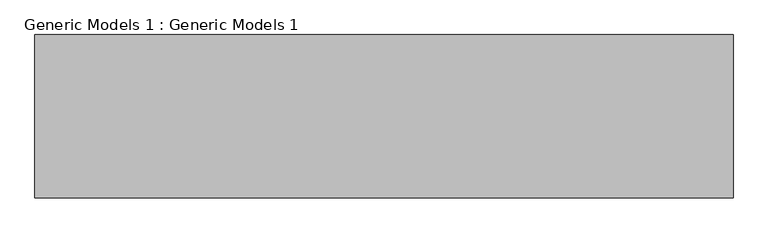
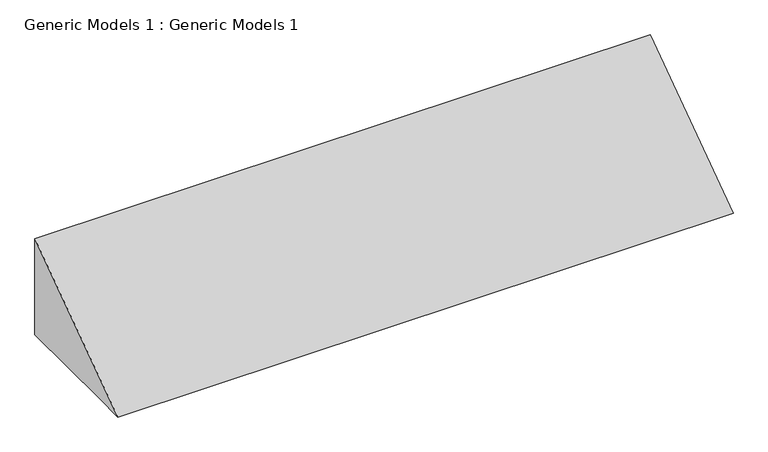
"""IFC4 building model written with IfcOpenShell, lengths in millimetres: proxy geometry, Generic Models 1 : Generic Models 1."""

from ifc_helpers import new_model, si_unit, frame, origin, place, context, project, spatial, polyline, outline, extrude, source, transform, mapped, element, save


def generic_models_1_generic_models_1_f97e06e3(model_context):
    return source(origin(), model_context, "Body", "SweptSolid", [
        extrude(outline(polyline([(-2756.7499863, 0.0), (-3188.5499863, 0.0), (-3315.5499863, 0.0), (-2756.7499863, 394.4470588), (-2756.7499863, 0.0)])), frame((-11589.0890533, 0.0, 0.0), z_axis=(1.0, 0.0, 0.0), x_axis=(0.0, 1.0, 0.0)), (0.0, 0.0, 1.0), 2390.9866667),
    ])


if __name__ == "__main__":
    model = new_model("IFC4")
    model_context = context("Model", 3, world=origin())
    ifc_project = project(units=[si_unit("LENGTHUNIT", "METRE", prefix="MILLI")], contexts=[model_context])
    site = spatial("IfcSite", under=ifc_project)
    building = spatial("IfcBuilding", under=site)
    placement = place(None, origin())
    generic_models_1_generic_models_1_shape = generic_models_1_generic_models_1_f97e06e3(model_context)
    element("IfcBuildingElementProxy", 1, Name="Generic Models 1 : Generic Models 1", ObjectType="Generic Models 1 : Generic Models 1", at=placement, inside=building, context=model_context, shape_type="MappedRepresentation", body=[
        mapped(generic_models_1_generic_models_1_shape, transform((0.0, 0.0, 0.0), x_axis=(1.0, 0.0, 0.0), y_axis=(0.0, 1.0, 0.0), z_axis=(0.0, 0.0, 1.0))),
    ])
    save(model, "model.ifc")

# Revit data of these elements
# Element 1 (IfcBuildingElementProxy, "Generic Models 1 : Generic Models 1")
#   Materials on its faces: "Tile, Porcelain, 4in"
# Materials
#   "Tile, Porcelain, 4in": class "Generic", colour RGB 89 87 158, transparency 0, Description = "Porcelain tile, 4\", white", Cost = 0
